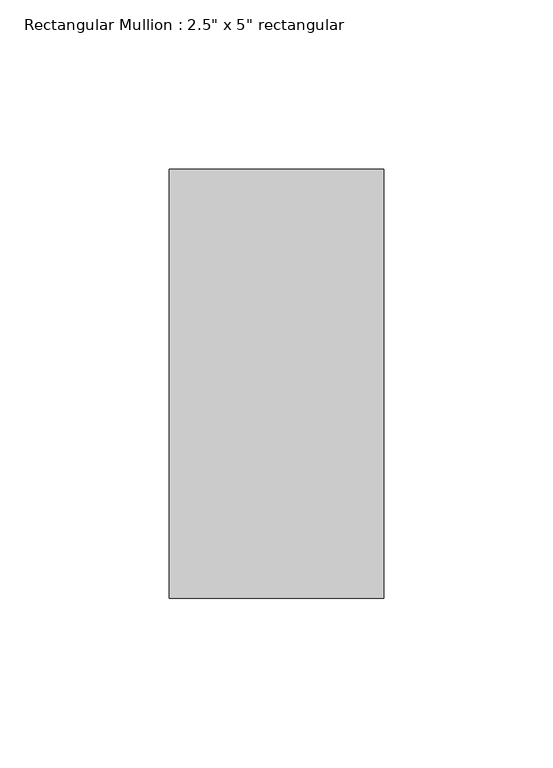
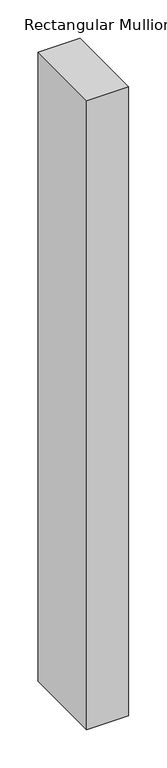
"""IFC4 building model written with IfcOpenShell, lengths in millimetres: member geometry."""

from ifc_helpers import new_model, si_unit, frame, origin, place, context, project, spatial, polyline, outline, extrude, source, transform, mapped, element, save


def member_b0389538(model_context):
    return source(origin(), model_context, "Body", "SweptSolid", [
        extrude(outline(polyline([(0.0, 63.5), (0.0, -63.5), (-63.5, -63.5), (-63.5, 63.5), (0.0, 63.5)])), frame((0.0, 0.0, -1003.2999998), z_axis=(0.0, 0.0, 1.0), x_axis=(1.0, 0.0, 0.0)), (0.0, 0.0, 1.0), 1003.2999998),
    ])


if __name__ == "__main__":
    model = new_model("IFC4")
    model_context = context("Model", 3, world=origin())
    ifc_project = project(units=[si_unit("LENGTHUNIT", "METRE", prefix="MILLI")], contexts=[model_context])
    site = spatial("IfcSite", under=ifc_project)
    building = spatial("IfcBuilding", under=site)
    placement = place(None, origin())
    member_shape = member_b0389538(model_context)
    element("IfcMember", 1, ObjectType="Rectangular Mullion : 2.5\" x 5\" rectangular", at=placement, inside=building, context=model_context, shape_type="MappedRepresentation", body=[
        mapped(member_shape, transform((0.0, 0.0, 0.0), x_axis=(1.0, 0.0, 0.0), y_axis=(0.0, 1.0, 0.0), z_axis=(0.0, 0.0, 1.0))),
    ])
    save(model, "model.ifc")

# Revit data of these elements
# Type "Rectangular Mullion : 2.5\" x 5\" rectangular"
#   built-in parameter 1007304 = 0.416667 (stored number, unit not read)
#   built-in parameter 1007301 = 0.104167 (stored number, unit not read)
#   built-in parameter 1007300 = 0.104167 (stored number, unit not read)
# Element 1 (IfcMember, "Rectangular Mullion : 2.5\" x 5\" rectangular")
#   Materials on its faces: "Aluminum"
# Materials
#   "Aluminum": class "Metal", colour RGB 247 247 247, transparency 0, Description = "Aluminum 6061", Cost = 0
